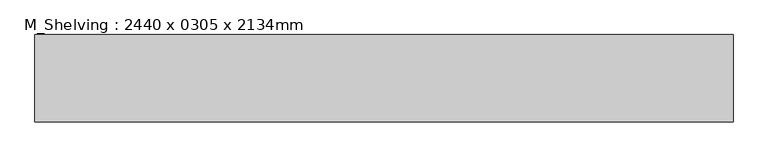
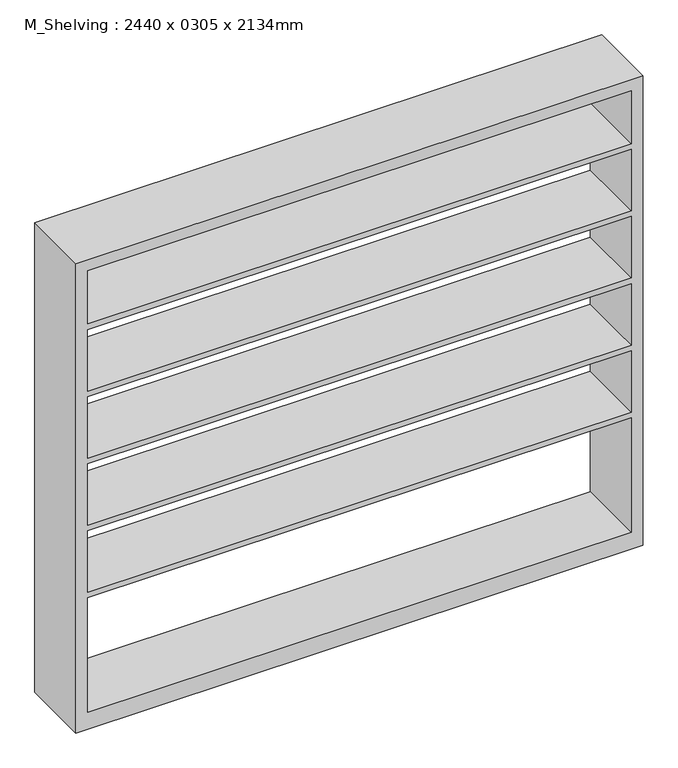
"""IFC4 building model written with IfcOpenShell, lengths in millimetres: furniture geometry, M_Shelving : 2440 x 0305 x 2134mm."""

from ifc_helpers import new_model, si_unit, frame, origin, place, context, project, spatial, polyline, outline, extrude, source, transform, mapped, element, save


def m_shelving_2440_x_0305_x_2134mm_59c1a9e4(model_context):
    return source(origin(), model_context, "Body", "SweptSolid", [
        extrude(outline(polyline([(0.0, 1220.0), (2134.0, 1220.0), (2134.0, -1220.0), (0.0, -1220.0), (0.0, 1220.0)]), holes=[polyline([(2083.2, 1169.2), (1841.8428571, 1169.2), (1841.8428571, -1169.2), (2083.2, -1169.2), (2083.2, 1169.2)]), polyline([(76.2, 1169.2), (76.2, -1169.2), (597.0142857, -1169.2), (597.0142857, 1169.2), (76.2, 1169.2)]), polyline([(1232.1285714, -1169.2), (1511.5857143, -1169.2), (1511.5857143, 1169.2), (1232.1285714, 1169.2), (1232.1285714, -1169.2)]), polyline([(1816.4428571, 1169.2), (1536.9857143, 1169.2), (1536.9857143, -1169.2), (1816.4428571, -1169.2), (1816.4428571, 1169.2)]), polyline([(1206.7285714, 1169.2), (927.2714286, 1169.2), (927.2714286, -1169.2), (1206.7285714, -1169.2), (1206.7285714, 1169.2)]), polyline([(901.8714286, 1169.2), (622.4142857, 1169.2), (622.4142857, -1169.2), (901.8714286, -1169.2), (901.8714286, 1169.2)])]), frame((0.0, -457.3, 0.0), z_axis=(0.0, 1.0, 0.0), x_axis=(0.0, 0.0, 1.0)), (0.0, 0.0, 1.0), 305.0),
    ])


if __name__ == "__main__":
    model = new_model("IFC4")
    model_context = context("Model", 3, world=origin())
    ifc_project = project(units=[si_unit("LENGTHUNIT", "METRE", prefix="MILLI")], contexts=[model_context])
    site = spatial("IfcSite", under=ifc_project)
    building = spatial("IfcBuilding", under=site)
    placement = place(None, origin())
    m_shelving_2440_x_0305_x_2134mm_shape = m_shelving_2440_x_0305_x_2134mm_59c1a9e4(model_context)
    element("IfcFurniture", 1, ObjectType="M_Shelving : 2440 x 0305 x 2134mm", at=placement, inside=building, context=model_context, shape_type="MappedRepresentation", body=[
        mapped(m_shelving_2440_x_0305_x_2134mm_shape, transform((0.0, 0.0, 0.0), x_axis=(1.0, 0.0, 0.0), y_axis=(0.0, 1.0, 0.0), z_axis=(0.0, 0.0, 1.0))),
    ])
    save(model, "model.ifc")

# Revit data of these elements
# Type "M_Shelving : 2440 x 0305 x 2134mm"
#   Depth = 305 mm
#   Height = 2134 mm
#   Width = 2440 mm
#   Material = Laminate, Ivory, Matte
#   Default Elevation = 0
# Element 1 (IfcFurniture, "M_Shelving : 2440 x 0305 x 2134mm")
#   Materials on its faces: "Laminate, Ivory, Matte"
# Materials
#   "Laminate, Ivory, Matte": class "Plastic", colour RGB 247 247 229, transparency 0, Description = "Plastic Laminate - Ivory, Matte", Cost = 0
